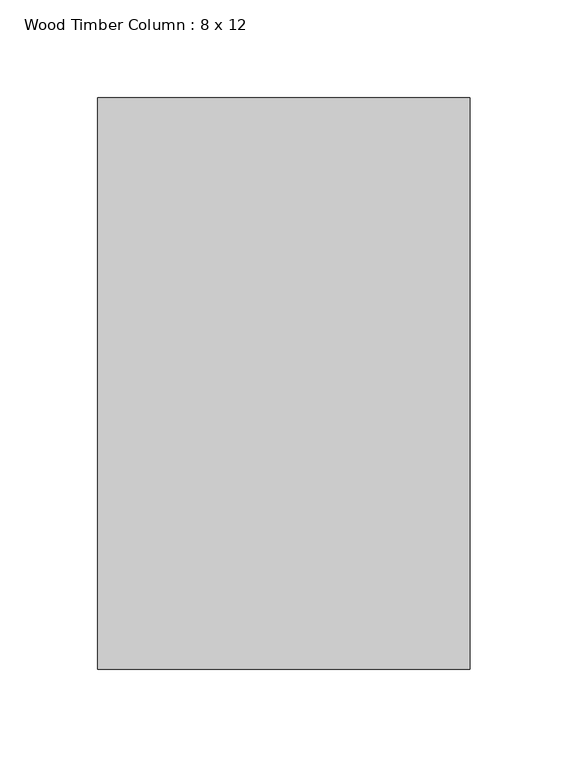
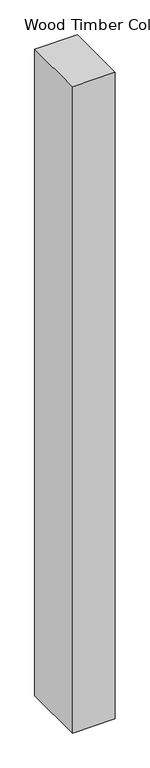
"""IFC4 building model written with IfcOpenShell, lengths in millimetres: column geometry, Wood Timber Column : 8 x 12."""

from ifc_helpers import new_model, si_unit, frame, origin, place, context, project, spatial, polyline, outline, extrude, source, transform, mapped, element, save


def wood_timber_column_8_x_12_7c9a4679(model_context):
    return source(origin(), model_context, "Body", "SweptSolid", [
        extrude(outline(polyline([(95.25, -146.05), (-95.25, -146.05), (-95.25, 146.05), (95.25, 146.05), (95.25, -146.05)])), frame((0.0, 0.0, 11845.2339631), z_axis=(0.0, 0.0, 1.0), x_axis=(1.0, 0.0, 0.0)), (0.0, 0.0, 1.0), 3048.0),
    ])


if __name__ == "__main__":
    model = new_model("IFC4")
    model_context = context("Model", 3, world=origin())
    ifc_project = project(units=[si_unit("LENGTHUNIT", "METRE", prefix="MILLI")], contexts=[model_context])
    site = spatial("IfcSite", under=ifc_project)
    building = spatial("IfcBuilding", under=site)
    placement = place(None, origin())
    wood_timber_column_8_x_12_shape = wood_timber_column_8_x_12_7c9a4679(model_context)
    element("IfcColumn", 1, ObjectType="Wood Timber Column : 8 x 12", at=placement, inside=building, context=model_context, shape_type="MappedRepresentation", body=[
        mapped(wood_timber_column_8_x_12_shape, transform((0.0, 0.0, 0.0), x_axis=(1.0, 0.0, 0.0), y_axis=(0.0, 1.0, 0.0), z_axis=(0.0, 0.0, 1.0))),
    ])
    save(model, "model.ifc")

# Revit data of these elements
# Type "Wood Timber Column : 8 x 12"
#   Assembly Code = "B1010200"
#   Depth = 0' - 11 1/2"
#   Width = 0' - 7 1/2"
#   Material = Softwood, Lumber
# Element 1 (IfcColumn, "Wood Timber Column : 8 x 12")
#   Materials on its faces: "Softwood, Lumber"
# Materials
#   "Softwood, Lumber": class "Wood", colour RGB 223 192 134, transparency 0, Description = "Pinus Echinata", Cost = 0
